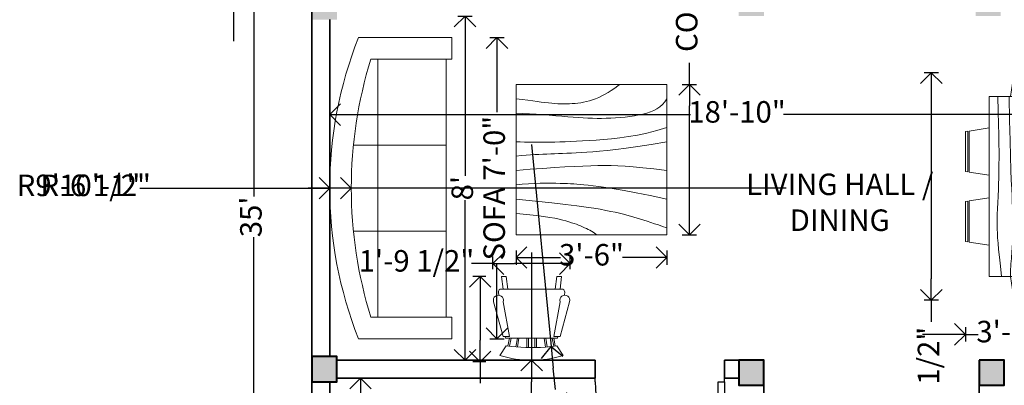
# Model space of a CAD drawing. Units: inches. Extents: x 261 to 714, y 97 to 573.
# Tile 2 of 5: x 266 to 541, y 286 to 388. Entities that reach past the tile are written whole.
import ezdxf

# ---------------------------------------------------------------- set-up
doc = ezdxf.new("R2010")
doc.units = ezdxf.units.IN
for name, color, linetype, lineweight in [('A-ANNO-DIMS', 2, 'Continuous', 18), ('A-AREA-IDEN', 7, 'Continuous', 25), ('A-COLS', 182, 'Continuous', 40), ('A-COLS-PATT', 172, 'Continuous', 13), ('A-DOOR', 182, 'Continuous', 25), ('A-FURN', 8, 'Continuous', 18), ('A-WALL', 182, 'Continuous', 35)]:
    doc.layers.add(name, color=color, linetype=linetype, lineweight=lineweight)
doc.styles.get("Standard").update_dxf_attribs({"font": 'arial.ttf'})
doc.dimstyles.new('ISO-25', dxfattribs={"dimtxt": 6, "dimasz": 6, "dimexe": 2, "dimexo": 2, "dimtad": 0, "dimdec": 1, "dimlunit": 3, "dimtxsty": 'Standard', "dimblk": 'OPEN90', "dimcen": 2.5, "dimclrd": 1, "dimclre": 1, "dimclrt": 1, "dimadec": 0, "dimazin": 0, "dimtfac": 1, "dimtdec": 1, "dimtmove": 0, "dimatfit": 3, "dimfxl": 2, "dimfxlon": 1, "dimarcsym": 0})

# ---------------------------------------------------------------- blocks, each defined once
blk = doc.blocks.new('*U4')
for p, q in [((0, 0), (0, -6)), ((36, 0), (36, -6))]:
    blk.add_line(p, q)
blk.add_lwpolyline([(0, 0), (0, 36), (1.75, 36), (1.75, 0)], close=True)
blk.add_arc((0, 0), 36, 0, 90)
blk = doc.blocks.new('_Open90')
at = {"color": 0, "linetype": 'ByBlock', "lineweight": -2}
for p, q in [((-0.5, 0.5), (0, 0)), ((0, 0), (-1, 0)), ((0, 0), (-0.5, -0.5))]:
    blk.add_line(p, q, dxfattribs=at)
blk = doc.blocks.new('*D15')
at = {"layer": 'A-ANNO-DIMS', "color": 0, "lineweight": -2, "transparency": 16777216}
for p, q in [((352.9, 361.16), (352.9, 359.16)), ((358.9, 361.16), (453.42, 361.16)), ((573.9, 361.16), (479.38, 361.16)), ((579.9, 361.16), (579.9, 359.16))]:
    blk.add_line(p, q, dxfattribs=at)
at = {"layer": 'Defpoints', "color": 0, "transparency": 16777216}
for p in [(352.9, 361.54), (579.9, 361.54), (579.9, 361.16)]:
    blk.add_point(p, dxfattribs=at)
at = {"layer": 'A-ANNO-DIMS', "color": 0, "lineweight": -2, "transparency": 16777216, "xscale": 6, "yscale": 6, "zscale": 6, "rotation": 180}
blk.add_blockref('_Open90', (352.9, 361.16), dxfattribs=at)
at = {"layer": 'A-ANNO-DIMS', "color": 0, "lineweight": -2, "transparency": 16777216, "xscale": 6, "yscale": 6, "zscale": 6}
blk.add_blockref('_Open90', (579.9, 361.16), dxfattribs=at)
at = {"layer": 'A-ANNO-DIMS', "color": 0, "transparency": 16777216, "insert": (466.4, 361.16), "char_height": 6, "attachment_point": 5}
blk.add_mtext('18\'-10"', dxfattribs=at)
blk = doc.blocks.new('*D16')
at = {"layer": 'A-ANNO-DIMS', "color": 0, "lineweight": -2, "transparency": 16777216}
for p, q in [((388.61, 388.66), (392.61, 388.66)), ((390.61, 382.66), (390.61, 344.05)), ((390.61, 298.66), (390.61, 337.27)), ((388.61, 292.66), (392.61, 292.66))]:
    blk.add_line(p, q, dxfattribs=at)
at = {"layer": 'Defpoints', "color": 0, "transparency": 16777216}
for p in [(378.75, 388.66), (378.75, 292.66), (390.61, 292.66)]:
    blk.add_point(p, dxfattribs=at)
at = {"layer": 'A-ANNO-DIMS', "color": 0, "lineweight": -2, "transparency": 16777216, "xscale": 6, "yscale": 6, "zscale": 6}
for p, rotation in [((390.61, 388.66), 90), ((390.61, 292.66), 270)]:
    blk.add_blockref('_Open90', p, dxfattribs=dict(at, rotation=rotation))
at = {"layer": 'A-ANNO-DIMS', "color": 0, "transparency": 16777216, "insert": (390.61, 340.66), "char_height": 6, "attachment_point": 5, "rotation": 90}
blk.add_mtext("8'", dxfattribs=at)
blk = doc.blocks.new('*D20')
at = {"layer": 'A-ANNO-DIMS', "color": 0, "lineweight": -2, "transparency": 16777216}
for p, q in [((363.48, 287.66), (359.48, 287.66)), ((361.48, 281.66), (361.48, 233.09)), ((361.48, 173.66), (361.48, 222.22)), ((363.48, 167.66), (359.48, 167.66))]:
    blk.add_line(p, q, dxfattribs=at)
at = {"layer": 'Defpoints', "color": 0, "transparency": 16777216}
for p in [(378.83, 287.66), (361.48, 167.66), (378.83, 167.66)]:
    blk.add_point(p, dxfattribs=at)
at = {"layer": 'A-ANNO-DIMS', "color": 0, "lineweight": -2, "transparency": 16777216, "xscale": 6, "yscale": 6, "zscale": 6}
for p, rotation in [((361.48, 287.66), 90), ((361.48, 167.66), 270)]:
    blk.add_blockref('_Open90', p, dxfattribs=dict(at, rotation=rotation))
at = {"layer": 'A-ANNO-DIMS', "color": 0, "transparency": 16777216, "insert": (361.48, 227.66), "char_height": 6, "attachment_point": 5, "rotation": 90}
blk.add_mtext("10'", dxfattribs=at)
blk = doc.blocks.new('Sofa - Roundback 7 ft.')
for p, q in [((-12.00002, -32.4421), (-12.00003, -6.5971)), ((11.99997, -32.4421), (11.99998, -6.5971)), ((-36.000027, -34), (-36.000027, -11.4696)), ((-35.999844, -13.3819), (35.9998, -13.3819)), ((35.99998, -34), (35.99998, -11.4696)), ((-36.000027, -32.4421), (35.99998, -32.4421))]:
    blk.add_line(p, q)
for points in [[(-36.000027, -34), (-42.000027, -34), (-42.000027, -8)], [(41.99998, -8), (41.99998, -34), (35.99998, -34)]]:
    blk.add_lwpolyline(points)
for centre, radius, start, end in [((0, -114.25), 114.25, 68.43141, 111.5686), ((-0.00001, -127.1968), 121.1968, 72.72033, 107.2797)]:
    blk.add_arc(centre, radius, start, end)
blk = doc.blocks.new('Table - Square Woodgrain 42 x 42 in.')
blk.add_line((0, -42), (42, -42))
for points in [[(0, -4), (1.704, -4.2172), (3.2358, -4.4188), (4.615, -4.604), (5.8615, -4.7721), (6.9951, -4.9224), (8.0357, -5.0541), (9.0031, -5.1667), (9.9171, -5.2594), (10.7951, -5.3316), (11.6445, -5.3836), (12.4702, -5.4157), (13.277, -5.4283), (14.0698, -5.4217), (14.8535, -5.3964), (15.6331, -5.3526), (16.4133, -5.2908), (17.1986, -5.2103), (17.9913, -5.1062), (18.793, -4.9727), (19.6056, -4.8038), (20.4307, -4.5937), (21.2701, -4.3365), (22.1256, -4.0262), (22.9989, -3.6571), (23.888, -3.2272), (24.7756, -2.7516), (25.6408, -2.2491), (26.4624, -1.7387), (27.2195, -1.2395), (27.891, -0.7703), (28.456, -0.3501), (28.8934, 0.002)], [(0, -42), (0, 0), (42, 0), (42, -42)], [(0, -8), (1.8203, -8.1001), (3.6741, -8.2149), (5.5411, -8.3408), (7.4011, -8.4741), (9.2339, -8.6112), (11.0193, -8.7484), (12.7371, -8.8821), (14.3671, -9.0086), (15.8954, -9.1246), (17.3337, -9.2278), (18.6997, -9.3159), (20.0116, -9.387), (21.2871, -9.4389), (22.5442, -9.4696), (23.8008, -9.477), (25.0749, -9.459), (26.3791, -9.4137), (27.7049, -9.3403), (29.0383, -9.2382), (30.3655, -9.1068), (31.6728, -8.9455), (32.9461, -8.7535), (34.1717, -8.5304), (35.3358, -8.2756), (36.4268, -7.9863), (37.443, -7.6521), (38.3849, -7.2603), (39.253, -6.7986), (40.048, -6.2542), (40.7705, -5.6147), (41.421, -4.8674), (42, -4)], [(42, -12), (39.1784, -12.8621), (36.4519, -13.5654), (33.8246, -14.1294), (31.3004, -14.5731), (28.8832, -14.9161), (26.577, -15.1775), (24.3858, -15.3768), (22.3136, -15.5332), (20.3622, -15.6632), (18.5254, -15.7718), (16.7947, -15.8612), (15.1618, -15.9338), (13.6183, -15.9916), (12.1558, -16.0369), (10.7659, -16.0718), (9.4403, -16.0987), (8.1703, -16.1191), (6.9461, -16.1325), (5.7577, -16.1377), (4.595, -16.1335), (3.4479, -16.1188), (2.3064, -16.0924), (1.1604, -16.0532), (0, -16)], [(42, -16), (37.6529, -16.7365), (33.8802, -17.329), (30.6179, -17.7961), (27.8015, -18.1561), (25.3668, -18.4275), (23.2497, -18.6288), (21.3859, -18.7785), (19.7111, -18.8949), (18.1693, -18.9939), (16.7375, -19.0795), (15.401, -19.1534), (14.1449, -19.217), (12.9544, -19.2717), (11.8148, -19.3191), (10.7113, -19.3606), (9.6291, -19.3976), (8.5534, -19.4323), (7.47, -19.4689), (6.3643, -19.5122), (5.222, -19.5672), (4.0288, -19.6386), (2.7703, -19.7313), (1.4321, -19.8501), (0, -20)], [(0, -24), (3.9243, -23.6805), (7.4766, -23.4138), (10.6891, -23.1954), (13.5943, -23.0205), (16.2247, -22.8847), (18.6125, -22.7832), (20.7903, -22.7116), (22.7903, -22.6651), (24.6563, -22.642), (26.4764, -22.6507), (28.35, -22.7024), (30.3766, -22.8084), (32.6555, -22.98), (35.2861, -23.2283), (38.3678, -23.5645), (42, -24)], [(42, -32), (37.392, -31.017), (33.4585, -30.2231), (30.1291, -29.5949), (27.3334, -29.109), (25.0009, -28.742), (23.0612, -28.4707), (21.4439, -28.2716), (20.0786, -28.1215), (18.8998, -28.0002), (17.8609, -27.9014), (16.9206, -27.8219), (16.0371, -27.7588), (15.1691, -27.709), (14.2748, -27.6693), (13.3128, -27.6368), (12.2415, -27.6083), (11.0295, -27.5824), (9.6867, -27.5643), (8.233, -27.5608), (6.6884, -27.5787), (5.0728, -27.6248), (3.4062, -27.7058), (1.7086, -27.8286), (0, -28)], [(0, -32), (5.4026, -32.5358), (9.9494, -33.019), (13.7424, -33.4553), (16.8834, -33.8505), (19.4743, -34.2106), (21.6171, -34.5413), (23.4136, -34.8486), (24.9657, -35.1382), (26.3614, -35.4156), (27.6332, -35.6841), (28.7995, -35.9467), (29.8788, -36.2064), (30.8897, -36.4661), (31.8507, -36.7288), (32.7802, -36.9973), (33.6968, -37.2747), (34.6175, -37.5635), (35.5531, -37.8651), (36.5128, -38.1805), (37.506, -38.5108), (38.5421, -38.8568), (39.6302, -39.2197), (40.7797, -39.6004), (42, -40)], [(0, -36), (3.0098, -36.2857), (5.5354, -36.5643), (7.6368, -36.8359), (9.374, -37.1009), (10.807, -37.3597), (11.9957, -37.6126), (13.0002, -37.8599), (13.8804, -38.102), (14.6874, -38.3393), (15.4365, -38.5729), (16.1338, -38.8041), (16.7858, -39.0341), (17.3987, -39.264), (17.9787, -39.4952), (18.5322, -39.7288), (19.0655, -39.9662), (19.5832, -40.2081), (20.0842, -40.4544), (20.5657, -40.7046), (21.0249, -40.9581), (21.459, -41.2144), (21.8653, -41.4731), (22.2409, -41.7335), (22.5831, -41.9951)]]:
    blk.add_lwpolyline(points)
blk = doc.blocks.new('Dining Set - 36 x 72 in.')
for p, q in [((-22.2343, 26.00059), (-23.4847, 17.99762)), ((-22.2304, 26), (-5.7608, 26)), ((-22, 27.5), (-22.1562, 26.50042)), ((-5.8416, 26.5), (-22.1534, 26.5)), ((-22, 27.5), (-6, 27.5)), ((-5.8437, 26.49966), (-6, 27.5)), ((-4.5152, 17.99762), (-5.7655, 25.99926)), ((5.7657, 26.00059), (4.5153, 17.99762)), ((5.7696, 26), (22.2392, 26)), ((6, 27.5), (5.8438, 26.50042)), ((22.1584, 26.5), (5.8466, 26.5)), ((6, 27.5), (22, 27.5)), ((22.1563, 26.49966), (22, 27.5)), ((23.4848, 17.99762), (22.2345, 25.99926)), ((36, 18), (-36, 18)), ((-36, 18), (-36, -18)), ((36, -18), (36, 18)), ((-45.5, 8), (-44.5004, 8.15617)), ((-45.5, 8), (-45.5, -8)), ((-44.5, -8.15843), (-44.5, 8.15338)), ((-44.0006, 8.23428), (-35.9976, 9.48474)), ((-44, 8.23041), (-44, -8.23915)), ((44.0006, 8.23428), (35.9976, 9.48474)), ((44, 8.23041), (44, -8.23915)), ((44.5, -8.15843), (44.5, 8.15338)), ((45.5, 8), (44.5005, 8.15617)), ((45.5, 8), (45.5, -8)), ((-44.4997, -8.15631), (-45.5, -8)), ((-35.9976, -9.48476), (-43.9993, -8.2345)), ((35.9976, -9.48476), (43.9993, -8.2345)), ((44.4997, -8.15631), (45.5, -8)), ((-36, -18), (36, -18)), ((-22.2343, -26.0006), (-23.4847, -17.99762)), ((-4.5152, -17.99762), (-5.7655, -25.99928)), ((5.7657, -26.0006), (4.5153, -17.99762)), ((23.4848, -17.99762), (22.2345, -25.99928)), ((-22.2304, -26), (-5.7608, -26)), ((-22, -27.5), (-22.1562, -26.50044)), ((-5.8416, -26.5), (-22.1534, -26.5)), ((-22, -27.5), (-6, -27.5)), ((-5.8437, -26.49967), (-6, -27.5)), ((5.7696, -26), (22.2392, -26)), ((6, -27.5), (5.8438, -26.50044)), ((22.1584, -26.5), (5.8466, -26.5)), ((6, -27.5), (22, -27.5)), ((22.1563, -26.49967), (22, -27.5))]:
    blk.add_line(p, q)
for points in [[(-36, 15), (-31.1772, 14.97754), (-26.8079, 14.91406), (-22.8538, 14.81543), (-19.276, 14.6875), (-16.0362, 14.53613), (-13.0957, 14.36718), (-10.4159, 14.18652), (-7.9583, 14), (-5.6904, 13.81315), (-3.6035, 13.63021), (-1.6954, 13.45508), (0.0365, 13.29166), (1.5945, 13.14388), (2.9811, 13.01562), (4.1988, 12.9108), (5.25, 12.83333), (6.1393, 12.78613), (6.8802, 12.76823), (7.4883, 12.77767), (7.9792, 12.8125), (8.3685, 12.87077), (8.6719, 12.95052), (8.9049, 13.0498), (9.0833, 13.16666), (9.2205, 13.29899), (9.3216, 13.44401), (9.3895, 13.59879), (9.4271, 13.76041), (9.4373, 13.92594), (9.4232, 14.09245), (9.3875, 14.257), (9.3333, 14.41666), (9.2638, 14.56917), (9.1836, 14.71484), (9.0975, 14.85465), (9.0104, 14.98958), (8.9272, 15.1206), (8.8529, 15.2487), (8.7922, 15.37483), (8.75, 15.5), (8.7305, 15.62467), (8.7344, 15.74739), (8.7617, 15.86621), (8.8125, 15.97916), (8.8867, 16.08431), (8.9844, 16.17968), (9.1055, 16.26334), (9.25, 16.33333), (9.4189, 16.38802), (9.6172, 16.42708), (9.8506, 16.45052), (10.125, 16.45833), (10.4463, 16.45052), (10.8203, 16.42708), (11.2529, 16.38802), (11.75, 16.33333), (12.3184, 16.26318), (12.9694, 16.17838), (13.7151, 16.07991), (14.5677, 15.96875), (15.5395, 15.84586), (16.6426, 15.71224), (17.8893, 15.56884), (19.2917, 15.41666), (20.859, 15.25667), (22.5879, 15.08984), (24.4721, 14.91715), (26.5052, 14.73958), (28.6809, 14.5581), (30.9929, 14.3737), (33.4347, 14.18733), (36, 14)], [(-36, 10), (-28.9766, 10.14274), (-23.1725, 10.20442), (-18.4241, 10.19775), (-14.5677, 10.13541), (-11.4399, 10.03011), (-8.877, 9.89453), (-6.7154, 9.74137), (-4.7917, 9.58333), (-2.9698, 9.43082), (-1.2246, 9.28515), (0.4415, 9.14534), (2.026, 9.01041), (3.5266, 8.87939), (4.9408, 8.7513), (6.266, 8.62516), (7.5, 8.5), (8.6411, 8.37549), (9.6914, 8.2539), (10.6538, 8.13818), (11.5312, 8.03125), (12.3267, 7.93603), (13.043, 7.85547), (13.6831, 7.79248), (14.25, 7.75), (14.7471, 7.7303), (15.1797, 7.73307), (15.5537, 7.75732), (15.875, 7.80208), (16.1494, 7.86637), (16.3828, 7.94922), (16.5811, 8.04964), (16.75, 8.16666), (16.8944, 8.29915), (17.0143, 8.44531), (17.1089, 8.60319), (17.1771, 8.77083), (17.218, 8.94629), (17.2305, 9.1276), (17.2137, 9.31282), (17.1667, 9.5), (17.0895, 9.6875), (16.987, 9.875), (16.8649, 10.0625), (16.7292, 10.25), (16.5856, 10.4375), (16.4401, 10.625), (16.2985, 10.8125), (16.1667, 11), (16.05, 11.18733), (15.9518, 11.3737), (15.8752, 11.5581), (15.8229, 11.73958), (15.798, 11.91715), (15.8034, 12.08984), (15.842, 12.25667), (15.9167, 12.41666), (16.0295, 12.56836), (16.1784, 12.70833), (16.3605, 12.83268), (16.5729, 12.9375), (16.8127, 13.01888), (17.0768, 13.07291), (17.3625, 13.0957), (17.6667, 13.08333), (17.9894, 13.03312), (18.3418, 12.94726), (18.7382, 12.82918), (19.1927, 12.68229), (19.7195, 12.51001), (20.3327, 12.31575), (21.0465, 12.10294), (21.875, 11.875), (22.8357, 11.63354), (23.959, 11.37304), (25.2786, 11.08618), (26.8282, 10.76562), (28.6414, 10.40405), (30.752, 9.99414), (33.1936, 9.52856), (36, 9)], [(-36, 5.5), (-30.7157, 5.3348), (-26.069, 5.20963), (-21.9946, 5.11767), (-18.4271, 5.05208), (-15.3009, 5.00602), (-12.5508, 4.97265), (-10.1112, 4.94515), (-7.9167, 4.91666), (-5.909, 4.88167), (-4.0586, 4.83984), (-2.3429, 4.79215), (-0.7396, 4.73958), (0.7739, 4.6831), (2.22, 4.6237), (3.6213, 4.56233), (5, 4.5), (6.373, 4.43782), (7.7344, 4.3776), (9.0723, 4.32129), (10.375, 4.27083), (11.6309, 4.22819), (12.8281, 4.19531), (13.9551, 4.17415), (15, 4.16666), (15.954, 4.17448), (16.819, 4.19791), (17.6001, 4.23698), (18.3021, 4.29166), (18.9299, 4.36198), (19.4883, 4.44791), (19.9823, 4.54948), (20.4167, 4.66666), (20.7969, 4.79899), (21.1302, 4.94401), (21.4245, 5.09879), (21.6875, 5.26041), (21.9271, 5.42594), (22.1511, 5.59245), (22.3672, 5.757), (22.5834, 5.91666), (22.8065, 6.06868), (23.0404, 6.21093), (23.2879, 6.34147), (23.5521, 6.45833), (23.8358, 6.55957), (24.142, 6.64323), (24.4735, 6.70735), (24.8334, 6.75), (25.2235, 6.76969), (25.642, 6.76692), (26.0858, 6.74267), (26.5521, 6.69791), (27.0379, 6.63362), (27.5404, 6.55078), (28.0565, 6.45036), (28.5834, 6.33333), (29.1242, 6.19987), (29.7071, 6.04687), (30.3661, 5.87044), (31.1354, 5.66666), (32.0493, 5.43164), (33.142, 5.16146), (34.4475, 4.85221), (36, 4.5)], [(-36, -1), (-30.7915, -0.6591), (-26.0195, -0.38216), (-21.6519, -0.16284), (-17.6563, 0.00521), (-14.0005, 0.12833), (-10.6523, 0.21289), (-7.5796, 0.26522), (-4.75, 0.29166), (-2.134, 0.29793), (0.2878, 0.28711), (2.5317, 0.26163), (4.6146, 0.22396), (6.5529, 0.17651), (8.3633, 0.12174), (10.0623, 0.06209), (11.6667, 0), (13.1899, -0.06201), (14.6341, -0.1211), (15.9982, -0.17432), (17.2813, -0.21875), (18.4823, -0.25147), (19.6003, -0.26953), (20.6343, -0.27002), (21.5834, -0.25), (22.4481, -0.20768), (23.2357, -0.14584), (23.9549, -0.06836), (24.6146, 0.02083), (25.2235, 0.11784), (25.7904, 0.21875), (26.3241, 0.31966), (26.8334, 0.41666), (27.3265, 0.50618), (27.8099, 0.58593), (28.2894, 0.65397), (28.7709, 0.70833), (29.2601, 0.74707), (29.763, 0.76823), (30.2855, 0.76985), (30.8334, 0.75), (31.4088, 0.70784), (31.9994, 0.64713), (32.589, 0.57275), (33.1615, 0.48958), (33.7008, 0.4025), (34.1908, 0.3164), (34.6153, 0.23616), (34.9584, 0.16666), (35.2099, 0.11165), (35.3848, 0.07031), (35.504, 0.04069), (35.5886, 0.02083), (35.6594, 0.00879), (35.7377, 0.0026), (35.8442, 0.00032), (36, 0)], [(-36, -6.5), (-27.1843, -6.31267), (-20.084, -6.1263), (-14.469, -5.9419), (-10.1094, -5.76042), (-6.7752, -5.58285), (-4.2363, -5.41016), (-2.2629, -5.24333), (-0.625, -5.08334), (0.8708, -4.93099), (2.2715, -4.78646), (3.5872, -4.64974), (4.8281, -4.52084), (6.0046, -4.39974), (7.127, -4.28646), (8.2053, -4.18099), (9.25, -4.08334), (10.2705, -3.99382), (11.2734, -3.91407), (12.2647, -3.84603), (13.25, -3.79167), (14.2354, -3.75293), (15.2266, -3.73177), (16.2295, -3.73015), (17.25, -3.75), (18.2912, -3.79248), (19.3451, -3.85547), (20.4009, -3.93604), (21.4479, -4.03125), (22.4754, -4.13819), (23.4727, -4.25391), (24.4289, -4.37549), (25.3334, -4.5), (26.1785, -4.62492), (26.9694, -4.74935), (27.7145, -4.87281), (28.4219, -4.99479), (29.1, -5.11483), (29.7572, -5.23242), (30.4016, -5.34709), (31.0417, -5.45834), (31.6837, -5.56437), (32.3262, -5.65821), (32.9658, -5.73153), (33.599, -5.77604), (34.2224, -5.78345), (34.8327, -5.74545), (35.4264, -5.65373), (36, -5.5)], [(-36, -10), (-26.4022, -9.81299), (-18.4675, -9.62891), (-11.9839, -9.45069), (-6.7396, -9.28125), (-2.5226, -9.12354), (0.8789, -8.98047), (3.6769, -8.85498), (6.0833, -8.75), (8.2767, -8.66765), (10.3021, -8.60677), (12.1712, -8.56543), (13.8958, -8.54167), (15.4876, -8.53353), (16.9583, -8.53907), (18.3197, -8.55632), (19.5834, -8.58334), (20.7616, -8.61841), (21.8685, -8.66081), (22.9188, -8.71004), (23.9271, -8.76563), (24.9081, -8.82707), (25.8763, -8.89388), (26.8465, -8.96558), (27.8334, -9.04167), (28.8474, -9.12118), (29.8828, -9.20117), (30.93, -9.27824), (31.9792, -9.34896), (33.0205, -9.40991), (34.0443, -9.45768), (35.0407, -9.48885), (36, -9.5)], [(-36, -14.5), (-30.0881, -14.33513), (-25.0332, -14.21224), (-20.7312, -14.12647), (-17.0781, -14.07292), (-13.97, -14.04671), (-11.3027, -14.04297), (-8.9724, -14.05681), (-6.875, -14.08334), (-4.9224, -14.11833), (-3.0905, -14.16016), (-1.3709, -14.20785), (0.2448, -14.26042), (1.7647, -14.3169), (3.1973, -14.3763), (4.5507, -14.43767), (5.8333, -14.5), (7.0554, -14.5621), (8.235, -14.62175), (9.3922, -14.67652), (10.5469, -14.72396), (11.7192, -14.76164), (12.929, -14.78711), (14.1965, -14.79794), (15.5417, -14.79167), (16.9933, -14.76424), (18.6152, -14.70508), (20.4804, -14.60197), (22.6615, -14.44271), (25.2312, -14.21509), (28.2624, -13.9069), (31.8277, -13.50594), (36, -13)]]:
    blk.add_lwpolyline(points)
blk = doc.blocks.new('Chair - Rocking')
for p, q in [((-8, -4.5), (-10, -1.5)), ((8, -4.5), (10, -1.5)), ((-7.5, -4.5), (-7, -7)), ((-6.5, -7), (-7.02225, -4.43)), ((-4.5, -7), (-4.96674, -4.19951)), ((-4, -7), (-4.40532, -4.16272)), ((-1.5, -4.05012), (-1.5, -7)), ((-1, -7), (-1, -4.05012)), ((1, -7), (1, -4.04655)), ((1.5, -4.05012), (1.5, -7)), ((4, -7), (4.40187, -4.18694)), ((4.5, -7), (4.96761, -4.19437)), ((6.5, -7), (7, -4.4057)), ((7.5, -4.5), (7, -7)), ((-9, -7.5), (-12, -18.49999)), ((-7, -7.5), (-9, -7.5)), ((-9, -18.49999), (-7, -7.5)), ((-8.23428, -6.99939), (-8.3093, -7.47958)), ((-8.23041, -7), (8.23915, -7)), ((7, -7.5), (9, -7.5)), ((9, -18.49999), (7, -7.5)), ((8.31071, -7.48854), (8.23449, -7.00073)), ((9, -7.5), (12, -18.49999)), ((-10.36644, -20.64523), (-10.5, -21.49999)), ((10.5, -21.49999), (10.3575, -20.58798)), ((-9, -22.49999), (-9.5, -26.49999)), ((0, -22.49999), (-9.5, -22.49999)), ((-8, -26.49999), (-7.5, -22.49999)), ((0, -22.49999), (9.5, -22.49999)), ((8, -26.49999), (7.5, -22.49999)), ((9, -22.49999), (9.5, -26.49999)), ((-9.5, -26.49999), (-8, -26.49999)), ((9.5, -26.49999), (8, -26.49999))]:
    blk.add_line(p, q)
for centre, radius, start, end in [((0, -34.08333), 34.08333, 72.93847, 107.0615), ((0, -68.25004), 64.25, 93.92211, 97.15267), ((0, -68.25004), 64.25, 82.84733, 93.92211), ((-10.5, -18.99999), 1.58114, 161.5651, 18.43495), ((10.5, -18.99999), 1.58114, 161.5651, 18.43495), ((-9.5, -21.49999), 1, 180, 270), ((9.5, -21.49999), 1, 270, 0)]:
    blk.add_arc(centre, radius, start, end)
blk = doc.blocks.new('*D36')
at = {"layer": 'A-ANNO-DIMS', "color": 0, "lineweight": -2, "transparency": 16777216}
for p, q in [((333.7, 542.66), (329.7, 542.66)), ((331.7, 536.66), (331.7, 338.37)), ((331.7, 128.66), (331.7, 326.94)), ((333.7, 122.66), (329.7, 122.66))]:
    blk.add_line(p, q, dxfattribs=at)
at = {"layer": 'Defpoints', "color": 0, "transparency": 16777216}
for p in [(347.9, 542.66), (331.7, 122.66), (347.9, 122.66)]:
    blk.add_point(p, dxfattribs=at)
at = {"layer": 'A-ANNO-DIMS', "color": 0, "lineweight": -2, "transparency": 16777216, "xscale": 6, "yscale": 6, "zscale": 6}
for p, rotation in [((331.7, 542.66), 90), ((331.7, 122.66), 270)]:
    blk.add_blockref('_Open90', p, dxfattribs=dict(at, rotation=rotation))
at = {"layer": 'A-ANNO-DIMS', "color": 0, "transparency": 16777216, "insert": (331.7, 332.66), "char_height": 6, "attachment_point": 5, "rotation": 90}
blk.add_mtext("35'", dxfattribs=at)
blk = doc.blocks.new('COLUMN-7IN-SQUARE')
blk.add_lwpolyline([(0, 7), (0, 2), (0, 0), (2, 0), (7, 0), (7, 2), (7, 7)], close=True)
blk = doc.blocks.new('*D45')
at = {"layer": 'A-ANNO-DIMS', "color": 1, "lineweight": -2, "transparency": 16777216}
for p, q in [((397.5, 382.66), (401.5, 382.66)), ((399.5, 376.66), (399.5, 361.82)), ((399.5, 304.66), (399.5, 319.5)), ((397.5, 298.66), (401.5, 298.66))]:
    blk.add_line(p, q, dxfattribs=at)
at = {"layer": 'Defpoints', "color": 0, "transparency": 16777216}
for p in [(386.9, 382.66), (399.5, 382.66), (386.9, 298.66)]:
    blk.add_point(p, dxfattribs=at)
at = {"layer": 'A-ANNO-DIMS', "color": 1, "lineweight": -2, "transparency": 16777216, "xscale": 6, "yscale": 6, "zscale": 6}
for p, rotation in [((399.5, 382.66), 90), ((399.5, 298.66), 270)]:
    blk.add_blockref('_Open90', p, dxfattribs=dict(at, rotation=rotation))
at = {"layer": 'A-ANNO-DIMS', "color": 1, "transparency": 16777216, "insert": (399.5, 340.66), "char_height": 6, "attachment_point": 5, "rotation": 90}
blk.add_mtext('SOFA 7\'-0"', dxfattribs=at)
blk = doc.blocks.new('*D46')
at = {"layer": 'A-ANNO-DIMS', "color": 1, "lineweight": -2, "transparency": 16777216}
for p, q in [((344.24, 395.26), (338.24, 395.26)), ((350.24, 393.26), (350.24, 397.26)), ((350.24, 395.26), (352.98, 395.26)), ((386.9, 395.26), (384.16, 395.26)), ((386.9, 393.26), (386.9, 397.26)), ((392.9, 395.26), (398.9, 395.26))]:
    blk.add_line(p, q, dxfattribs=at)
at = {"layer": 'Defpoints', "color": 0, "transparency": 16777216}
for p in [(350.24, 395.26), (350.24, 382.66), (386.9, 382.66)]:
    blk.add_point(p, dxfattribs=at)
at = {"layer": 'A-ANNO-DIMS', "color": 1, "lineweight": -2, "transparency": 16777216, "xscale": 6, "yscale": 6, "zscale": 6}
blk.add_blockref('_Open90', (350.24, 395.26), dxfattribs=at)
at = {"layer": 'A-ANNO-DIMS', "color": 1, "lineweight": -2, "transparency": 16777216, "xscale": 6, "yscale": 6, "zscale": 6, "rotation": 180}
blk.add_blockref('_Open90', (386.9, 395.26), dxfattribs=at)
at = {"layer": 'A-ANNO-DIMS', "color": 1, "transparency": 16777216, "insert": (368.57, 395.26), "char_height": 6, "attachment_point": 5}
blk.add_mtext('3\'-0 1/2"', dxfattribs=at)
blk = doc.blocks.new('*D47')
at = {"layer": 'A-ANNO-DIMS', "color": 1, "lineweight": -2, "transparency": 16777216}
for p, q in [((453.15, 369.61), (453.15, 375.61)), ((451.15, 369.61), (455.15, 369.61)), ((453.15, 333.6), (453.15, 363.61)), ((451.15, 327.6), (455.15, 327.6))]:
    blk.add_line(p, q, dxfattribs=at)
at = {"layer": 'Defpoints', "color": 0, "transparency": 16777216}
for p in [(446.85, 369.61), (453.15, 369.61), (446.85, 327.6)]:
    blk.add_point(p, dxfattribs=at)
at = {"layer": 'A-ANNO-DIMS', "color": 1, "lineweight": -2, "transparency": 16777216, "xscale": 6, "yscale": 6, "zscale": 6}
for p, rotation in [((453.15, 369.61), 90), ((453.15, 327.6), 270)]:
    blk.add_blockref('_Open90', p, dxfattribs=dict(at, rotation=rotation))
at = {"layer": 'A-ANNO-DIMS', "color": 1, "transparency": 16777216, "insert": (453.15, 416.77), "char_height": 6, "attachment_point": 5, "rotation": 90}
blk.add_mtext('COFFEE TABLE 3\'-6"', dxfattribs=at)
blk = doc.blocks.new('*D48')
at = {"layer": 'A-ANNO-DIMS', "color": 1, "lineweight": -2, "transparency": 16777216}
for p, q in [((404.85, 323.3), (404.85, 319.3)), ((410.85, 321.3), (417.25, 321.3)), ((440.85, 321.3), (434.45, 321.3)), ((446.85, 323.3), (446.85, 319.3))]:
    blk.add_line(p, q, dxfattribs=at)
at = {"layer": 'Defpoints', "color": 0, "transparency": 16777216}
for p in [(404.85, 327.6), (446.85, 327.6), (446.85, 321.3)]:
    blk.add_point(p, dxfattribs=at)
at = {"layer": 'A-ANNO-DIMS', "color": 1, "lineweight": -2, "transparency": 16777216, "xscale": 6, "yscale": 6, "zscale": 6, "rotation": 180}
blk.add_blockref('_Open90', (404.85, 321.3), dxfattribs=at)
at = {"layer": 'A-ANNO-DIMS', "color": 1, "lineweight": -2, "transparency": 16777216, "xscale": 6, "yscale": 6, "zscale": 6}
blk.add_blockref('_Open90', (446.85, 321.3), dxfattribs=at)
at = {"layer": 'A-ANNO-DIMS', "color": 1, "transparency": 16777216, "insert": (425.85, 321.3), "char_height": 6, "attachment_point": 5}
blk.add_mtext('3\'-6"', dxfattribs=at)
blk = doc.blocks.new('*D51')
at = {"layer": 'A-ANNO-DIMS', "color": 1, "lineweight": -2, "transparency": 16777216}
for p, q in [((522.54, 372.81), (518.54, 372.81)), ((520.54, 366.81), (520.54, 315.39)), ((522.54, 309.39), (518.54, 309.39)), ((520.54, 309.39), (520.54, 303.39))]:
    blk.add_line(p, q, dxfattribs=at)
at = {"layer": 'Defpoints', "color": 0, "transparency": 16777216}
for p in [(530.06, 372.81), (520.54, 309.39), (530.06, 309.39)]:
    blk.add_point(p, dxfattribs=at)
at = {"layer": 'A-ANNO-DIMS', "color": 1, "lineweight": -2, "transparency": 16777216, "xscale": 6, "yscale": 6, "zscale": 6}
for p, rotation in [((520.54, 372.81), 90), ((520.54, 309.39), 270)]:
    blk.add_blockref('_Open90', p, dxfattribs=dict(at, rotation=rotation))
at = {"layer": 'A-ANNO-DIMS', "color": 1, "transparency": 16777216, "insert": (520.54, 262.8), "char_height": 6, "attachment_point": 5, "rotation": 90}
blk.add_mtext('DINING SET 5\'-3 1/2"', dxfattribs=at)
blk = doc.blocks.new('*D52')
at = {"layer": 'A-ANNO-DIMS', "color": 1, "lineweight": -2, "transparency": 16777216}
for p, q in [((530.06, 301.87), (530.06, 297.87)), ((568.39, 301.87), (568.39, 297.87)), ((524.06, 299.87), (518.06, 299.87)), ((530.06, 299.87), (533.63, 299.87)), ((568.39, 299.87), (564.81, 299.87)), ((574.39, 299.87), (580.39, 299.87))]:
    blk.add_line(p, q, dxfattribs=at)
at = {"layer": 'Defpoints', "color": 0, "transparency": 16777216}
for p in [(530.06, 309.39), (568.39, 309.39), (568.39, 299.87)]:
    blk.add_point(p, dxfattribs=at)
at = {"layer": 'A-ANNO-DIMS', "color": 1, "lineweight": -2, "transparency": 16777216, "xscale": 6, "yscale": 6, "zscale": 6}
blk.add_blockref('_Open90', (530.06, 299.87), dxfattribs=at)
at = {"layer": 'A-ANNO-DIMS', "color": 1, "lineweight": -2, "transparency": 16777216, "xscale": 6, "yscale": 6, "zscale": 6, "rotation": 180}
blk.add_blockref('_Open90', (568.39, 299.87), dxfattribs=at)
at = {"layer": 'A-ANNO-DIMS', "color": 1, "transparency": 16777216, "insert": (549.22, 299.87), "char_height": 6, "attachment_point": 5}
blk.add_mtext('3\'-2 1/2"', dxfattribs=at)
blk = doc.blocks.new('*D53')
at = {"layer": 'A-ANNO-DIMS', "color": 1, "lineweight": -2, "transparency": 16777216}
for p, q in [((396.37, 316.03), (392.8, 316.03)), ((394.8, 310.03), (394.8, 298.22)), ((396.37, 292.22), (392.8, 292.22)), ((394.8, 292.22), (394.8, 286.22))]:
    blk.add_line(p, q, dxfattribs=at)
at = {"layer": 'Defpoints', "color": 0, "transparency": 16777216}
for p in [(398.37, 316.03), (394.8, 292.22), (398.37, 292.22)]:
    blk.add_point(p, dxfattribs=at)
at = {"layer": 'A-ANNO-DIMS', "color": 1, "lineweight": -2, "transparency": 16777216, "xscale": 6, "yscale": 6, "zscale": 6}
for p, rotation in [((394.8, 316.03), 90), ((394.8, 292.22), 270)]:
    blk.add_blockref('_Open90', p, dxfattribs=dict(at, rotation=rotation))
at = {"layer": 'A-ANNO-DIMS', "color": 1, "transparency": 16777216, "insert": (394.8, 242.84), "char_height": 6, "attachment_point": 5, "rotation": 90}
blk.add_mtext('ROCKING CHAIR 2\'-0"', dxfattribs=at)
blk = doc.blocks.new('*D54')
at = {"layer": 'A-ANNO-DIMS', "color": 1, "lineweight": -2, "transparency": 16777216}
for p, q in [((398.37, 318.03), (398.37, 321.6)), ((419.93, 318.03), (419.93, 321.6)), ((398.37, 319.6), (392.37, 319.6)), ((413.93, 319.6), (404.37, 319.6))]:
    blk.add_line(p, q, dxfattribs=at)
at = {"layer": 'Defpoints', "color": 0, "transparency": 16777216}
for p in [(398.37, 319.6), (398.37, 316.03), (419.93, 316.03)]:
    blk.add_point(p, dxfattribs=at)
at = {"layer": 'A-ANNO-DIMS', "color": 1, "lineweight": -2, "transparency": 16777216, "xscale": 6, "yscale": 6, "zscale": 6, "rotation": 180}
blk.add_blockref('_Open90', (398.37, 319.6), dxfattribs=at)
at = {"layer": 'A-ANNO-DIMS', "color": 1, "lineweight": -2, "transparency": 16777216, "xscale": 6, "yscale": 6, "zscale": 6}
blk.add_blockref('_Open90', (419.93, 319.6), dxfattribs=at)
at = {"layer": 'A-ANNO-DIMS', "color": 1, "transparency": 16777216, "insert": (377.07, 319.6), "char_height": 6, "attachment_point": 5}
blk.add_mtext('1\'-9 1/2"', dxfattribs=at)
blk = doc.blocks.new('*D61')
at = {"layer": 'A-ANNO-DIMS', "color": 1, "lineweight": -2, "transparency": 16777216}
for p, q in [((354.9, 102.81), (354.9, 98.81)), ((426.9, 102.81), (426.9, 98.81)), ((360.9, 100.81), (382.29, 100.81)), ((420.9, 100.81), (399.52, 100.81))]:
    blk.add_line(p, q, dxfattribs=at)
at = {"layer": 'Defpoints', "color": 0, "transparency": 16777216}
for p in [(354.9, 287.66), (426.9, 287.66), (426.9, 100.81)]:
    blk.add_point(p, dxfattribs=at)
at = {"layer": 'A-ANNO-DIMS', "color": 1, "lineweight": -2, "transparency": 16777216, "xscale": 6, "yscale": 6, "zscale": 6, "rotation": 180}
blk.add_blockref('_Open90', (354.9, 100.81), dxfattribs=at)
at = {"layer": 'A-ANNO-DIMS', "color": 1, "lineweight": -2, "transparency": 16777216, "xscale": 6, "yscale": 6, "zscale": 6}
blk.add_blockref('_Open90', (426.9, 100.81), dxfattribs=at)
at = {"layer": 'A-ANNO-DIMS', "color": 1, "transparency": 16777216, "insert": (390.9, 100.81), "char_height": 6, "attachment_point": 5}
blk.add_mtext('6\'-0"', dxfattribs=at)
blk = doc.blocks.new('*D62')
at = {"layer": 'A-ANNO-DIMS', "color": 1, "lineweight": -2, "transparency": 16777216}
for p, q in [((426.9, 102.81), (426.9, 98.81)), ((462.9, 102.81), (462.9, 98.81)), ((432.9, 100.81), (436.31, 100.81)), ((456.9, 100.81), (453.5, 100.81))]:
    blk.add_line(p, q, dxfattribs=at)
at = {"layer": 'Defpoints', "color": 0, "transparency": 16777216}
for p in [(426.9, 287.66), (462.9, 287.66), (462.9, 100.81)]:
    blk.add_point(p, dxfattribs=at)
at = {"layer": 'A-ANNO-DIMS', "color": 1, "lineweight": -2, "transparency": 16777216, "xscale": 6, "yscale": 6, "zscale": 6, "rotation": 180}
blk.add_blockref('_Open90', (426.9, 100.81), dxfattribs=at)
at = {"layer": 'A-ANNO-DIMS', "color": 1, "lineweight": -2, "transparency": 16777216, "xscale": 6, "yscale": 6, "zscale": 6}
blk.add_blockref('_Open90', (462.9, 100.81), dxfattribs=at)
at = {"layer": 'A-ANNO-DIMS', "color": 1, "transparency": 16777216, "insert": (444.9, 100.81), "char_height": 6, "attachment_point": 5}
blk.add_mtext('3\'-0"', dxfattribs=at)
blk = doc.blocks.new('*D74')
at = {"layer": 'A-ANNO-DIMS', "color": 1, "lineweight": -2, "transparency": 16777216}
for p, q in [((326.05, 417.65), (326.05, 423.65)), ((328.05, 411.65), (324.05, 411.65)), ((326.05, 411.65), (326.05, 410.97)), ((328.05, 393.66), (324.05, 393.66)), ((326.05, 393.66), (326.05, 394.34)), ((326.05, 387.66), (326.05, 381.66))]:
    blk.add_line(p, q, dxfattribs=at)
at = {"layer": 'Defpoints', "color": 0, "transparency": 16777216}
for p in [(326.05, 411.65), (417.18, 411.65), (417.18, 393.66)]:
    blk.add_point(p, dxfattribs=at)
at = {"layer": 'A-ANNO-DIMS', "color": 1, "lineweight": -2, "transparency": 16777216, "xscale": 6, "yscale": 6, "zscale": 6}
for p, rotation in [((326.05, 411.65), 270), ((326.05, 393.66), 90)]:
    blk.add_blockref('_Open90', p, dxfattribs=dict(at, rotation=rotation))
at = {"layer": 'A-ANNO-DIMS', "color": 1, "transparency": 16777216, "insert": (326.05, 402.65), "char_height": 6, "attachment_point": 5, "rotation": 90}
blk.add_mtext('1\'-6"', dxfattribs=at)
blk = doc.blocks.new('*D79')
at = {"layer": 'A-ANNO-DIMS', "color": 1, "lineweight": -2, "transparency": 16777216}
for p, q in [((299.99, 340.66), (352.9, 340.66)), ((480.1, 340.66), (358.9, 340.66))]:
    blk.add_line(p, q, dxfattribs=at)
at = {"layer": 'Defpoints', "color": 0, "transparency": 16777216}
for p in [(358.9, 340.66), (480.1, 340.66)]:
    blk.add_point(p, dxfattribs=at)
at = {"layer": 'A-ANNO-DIMS', "color": 1, "lineweight": -2, "transparency": 16777216, "xscale": 6, "yscale": 6, "zscale": 6, "rotation": 0.0001238604833855}
blk.add_blockref('_Open90', (358.9, 340.66), dxfattribs=at)
at = {"layer": 'A-ANNO-DIMS', "color": 1, "transparency": 16777216, "insert": (286.19, 340.66), "char_height": 6, "attachment_point": 5, "rotation": 0.0001}
blk.add_mtext('R10\'-1"', dxfattribs=at)
blk = doc.blocks.new('*D80')
at = {"layer": 'A-ANNO-DIMS', "color": 1, "lineweight": -2, "transparency": 16777216}
for p, q in [((302.82, 340.66), (346.9, 340.66)), ((467.15, 340.66), (352.9, 340.66))]:
    blk.add_line(p, q, dxfattribs=at)
at = {"layer": 'Defpoints', "color": 0, "transparency": 16777216}
for p in [(352.9, 340.66), (467.15, 340.66)]:
    blk.add_point(p, dxfattribs=at)
at = {"layer": 'A-ANNO-DIMS', "color": 1, "lineweight": -2, "transparency": 16777216, "xscale": 6, "yscale": 6, "zscale": 6, "rotation": 0.0001364065822672}
blk.add_blockref('_Open90', (352.9, 340.66), dxfattribs=at)
at = {"layer": 'A-ANNO-DIMS', "color": 1, "transparency": 16777216, "insert": (284.35, 340.66), "char_height": 6, "attachment_point": 5, "rotation": 0.0001}
blk.add_mtext('R9\'-6 1/2"', dxfattribs=at)
blk = doc.blocks.new('*D81')
at = {"layer": 'A-ANNO-DIMS', "color": 1, "lineweight": -2, "transparency": 16777216}
for p, q in [((409.15, 352.86), (414.62, 296.45)), ((415.78, 284.51), (415.2, 290.48))]:
    blk.add_line(p, q, dxfattribs=at)
at = {"layer": 'Defpoints', "color": 0, "transparency": 16777216}
for p in [(409.15, 352.86), (414.62, 296.45)]:
    blk.add_point(p, dxfattribs=at)
at = {"layer": 'A-ANNO-DIMS', "color": 1, "lineweight": -2, "transparency": 16777216, "xscale": 6, "yscale": 6, "zscale": 6, "rotation": 95.53759783759804}
blk.add_blockref('_Open90', (414.62, 296.45), dxfattribs=at)
at = {"layer": 'A-ANNO-DIMS', "color": 1, "transparency": 16777216, "insert": (418.19, 259.66), "char_height": 6, "attachment_point": 5, "rotation": 275.5376}
blk.add_mtext('2X R4\'-8 1/2"', dxfattribs=at)
blk = doc.blocks.new('*D82')
at = {"layer": 'A-ANNO-DIMS', "color": 1, "lineweight": -2, "transparency": 16777216}
for p, q in [((409.15, 322.72), (409.15, 292.66)), ((409.15, 280.66), (409.15, 286.66))]:
    blk.add_line(p, q, dxfattribs=at)
at = {"layer": 'Defpoints', "color": 0, "transparency": 16777216}
for p in [(409.15, 322.72), (409.15, 292.66)]:
    blk.add_point(p, dxfattribs=at)
at = {"layer": 'A-ANNO-DIMS', "color": 1, "lineweight": -2, "transparency": 16777216, "xscale": 6, "yscale": 6, "zscale": 6, "rotation": 90.00021153640085}
blk.add_blockref('_Open90', (409.15, 292.66), dxfattribs=at)
at = {"layer": 'A-ANNO-DIMS', "color": 1, "transparency": 16777216, "insert": (409.15, 269.19), "char_height": 6, "attachment_point": 5, "rotation": 270.0002}
blk.add_mtext('R2\'-6"', dxfattribs=at)

msp = doc.modelspace()

# ---------------------------------------------------------------- hatches: boundary and pattern name
at = {"layer": 'A-COLS-PATT'}
h = msp.add_hatch(color=256, dxfattribs=at)
h.dxf.hatch_style = 1
h.paths.add_polyline_path([(354.9, 542.66), (347.9, 542.66), (347.9, 535.66), (354.9, 535.66)])
h.paths.add_polyline_path([(539.9, 542.66), (532.9, 542.66), (532.9, 537.66), (532.9, 535.66), (534.9, 535.66), (539.9, 535.66), (539.9, 537.66)])
h.paths.add_polyline_path([(474.9, 542.66), (467.9, 542.66), (467.9, 537.66), (467.9, 535.66), (469.9, 535.66), (474.9, 535.66), (474.9, 537.66)])
h.paths.add_polyline_path([(659.9, 542.66), (652.9, 542.66), (652.9, 537.66), (652.9, 535.66), (654.9, 535.66), (659.9, 535.66)])
h.paths.add_polyline_path([(659.9, 395.66), (652.88, 395.66), (652.88, 390.66), (652.88, 388.66), (654.88, 388.66), (659.9, 388.66)])
h.paths.add_polyline_path([(539.9, 395.66), (532.9, 395.66), (532.9, 390.66), (532.9, 388.66), (534.9, 388.66), (539.9, 388.66), (539.9, 390.66)])
h.paths.add_polyline_path([(473.9, 395.66), (466.9, 395.66), (466.9, 394.66), (466.9, 388.66), (473.9, 388.66)])
h.paths.add_polyline_path([(354.9, 394.66), (347.9, 394.66), (347.9, 389.66), (347.9, 387.66), (349.9, 387.66), (354.9, 387.66), (354.9, 389.66)])
h.paths.add_polyline_path([(540.9, 292.66), (533.9, 292.66), (533.9, 287.66), (533.9, 285.66), (535.9, 285.66), (540.9, 285.66), (540.9, 287.66)])
h.paths.add_polyline_path([(659.9, 294.66), (652.88, 294.66), (652.88, 289.66), (652.88, 287.66), (654.88, 287.66), (659.9, 287.66)])
h.paths.add_polyline_path([(473.9, 292.66), (466.9, 292.66), (466.9, 287.66), (466.9, 285.66), (468.9, 285.66), (473.9, 285.66), (473.9, 287.66)])
h.paths.add_polyline_path([(354.9, 293.66), (347.9, 293.66), (347.9, 288.66), (347.9, 286.66), (349.9, 286.66), (354.9, 286.66), (354.9, 288.66)])
h.paths.add_polyline_path([(354.9, 129.66), (347.9, 129.66), (347.9, 124.66), (347.9, 122.66), (349.9, 122.66), (354.9, 122.66), (354.9, 124.66)])
h.paths.add_polyline_path([(354.9, 168.66), (347.9, 168.66), (347.9, 163.66), (347.9, 161.66), (349.9, 161.66), (354.9, 161.66), (354.9, 163.66)])
h.paths.add_polyline_path([(473.9, 169.69), (466.95, 169.69), (466.95, 164.69), (466.95, 162.69), (468.95, 162.69), (473.9, 162.69)])
h.paths.add_polyline_path([(475.9, 129.66), (468.9, 129.66), (468.9, 124.66), (468.9, 122.66), (470.9, 122.66), (475.9, 122.66), (475.9, 124.66)])
h.paths.add_polyline_path([(540.9, 129.66), (533.9, 129.66), (533.9, 124.66), (533.9, 122.66), (535.9, 122.66), (540.9, 122.66), (540.9, 124.66)])
h.paths.add_polyline_path([(540.9, 169.66), (533.9, 169.66), (533.9, 164.66), (533.9, 162.66), (535.9, 162.66), (540.9, 162.66), (540.9, 164.66)])
h.paths.add_polyline_path([(659.9, 169.66), (652.9, 169.66), (652.9, 164.66), (652.9, 162.66), (654.9, 162.66), (659.9, 162.66)])
h.paths.add_polyline_path([(659.9, 129.66), (652.9, 129.66), (652.9, 124.66), (652.9, 122.66), (654.9, 122.66), (659.9, 122.66)])

# ---------------------------------------------------------------- linework, layer by layer
at = {"layer": 'A-WALL'}
for p, q in [((347.9, 542.66), (347.9, 122.66)), ((352.9, 387.66), (352.9, 293.66)), ((426.9, 292.66), (354.9, 292.66)), ((426.9, 292.66), (426.9, 287.66)), ((473.9, 292.66), (462.9, 292.66)), ((462.9, 292.66), (462.9, 287.66)), ((473.9, 292.66), (473.9, 129.66)), ((533.9, 292.66), (538.9, 292.66)), ((533.9, 292.66), (533.9, 127.66)), ((352.9, 286.66), (352.9, 168.66)), ((426.9, 287.66), (354.9, 287.66)), ((466.9, 287.66), (462.9, 287.66))]:
    msp.add_line(p, q, dxfattribs=at)

# ---------------------------------------------------------------- block references
at = {"layer": 'A-COLS'}
for p in [(347.9, 286.66), (466.9, 285.66), (533.9, 285.66)]:
    msp.add_blockref('COLUMN-7IN-SQUARE', p, dxfattribs=at)
at = {"layer": 'A-DOOR', "rotation": 180}
msp.add_blockref('*U4', (462.9, 286.66), dxfattribs=at)
at = {"layer": 'A-FURN', "rotation": 90}
msp.add_blockref('Sofa - Roundback 7 ft.', (352.9, 340.66), dxfattribs=at)
at = {"layer": 'A-FURN'}
for name, p, xscale, yscale, zscale, rotation in [('Dining Set - 36 x 72 in.', (549.22, 341.1), 0.6969524783132904, 0.6969524783132904, 0.6969524783132904, 270), ('Chair - Rocking', (409.15, 292.66), 0.8821013146512623, 0.8821013146512623, 0.8821013146512623, 180)]:
    msp.add_blockref(name, p, dxfattribs=dict(at, xscale=xscale, yscale=yscale, zscale=zscale, rotation=rotation))
msp.add_blockref('Table - Square Woodgrain 42 x 42 in.', (404.85, 369.6), dxfattribs=at)

# ---------------------------------------------------------------- texts
at = {"layer": 'A-AREA-IDEN', "insert": (464.61, 344.72), "char_height": 6, "attachment_point": 1}
msp.add_mtext_dynamic_manual_height_columns('\\pxqc;{LIVING HALL / \\PDINING}', width=60.8654, gutter_width=12.5, heights=[0], dxfattribs=at)

# ---------------------------------------------------------------- dimensions: what is measured, and where the dimension line sits
at = {"layer": 'A-ANNO-DIMS'}
for base, p1, p2, angle, override, picture, middle in [((331.7, 122.66), (347.9, 542.66), (347.9, 122.66), 90, {"dimclrd": 0, "dimclre": 0, "dimclrt": 0}, '*D36', (331.7, 332.66)), ((326.05, 411.65), (417.18, 393.66), (417.18, 411.65), 90, {"dimdec": 1, "dimlfac": 1, "dimrnd": 0, "dimzin": 1, "dimdsep": 46, "dimlunit": 4, "dimfrac": 2}, '*D74', (326.05, 402.65)), ((350.24, 395.26), (386.9, 382.66), (350.24, 382.66), 180, {"dimdec": 1, "dimlfac": 1, "dimrnd": 0, "dimzin": 1, "dimdsep": 46, "dimlunit": 4, "dimfrac": 2}, '*D46', (368.57, 395.26)), ((398.37, 319.6), (419.93, 316.03), (398.37, 316.03), 180, {"dimdec": 1, "dimlfac": 1, "dimrnd": 0, "dimzin": 1, "dimdsep": 46, "dimlunit": 4, "dimfrac": 2}, '*D54', (377.07, 319.6)), ((361.48, 167.66), (378.83, 287.66), (378.83, 167.66), 90, {"dimclrd": 0, "dimclre": 0, "dimclrt": 0}, '*D20', (361.48, 227.66))]:
    dim = msp.add_linear_dim(base=base, p1=p1, p2=p2, angle=angle, dimstyle='ISO-25', override=override, dxfattribs=at)
    dim.commit()
    dim.dimension.update_dxf_attribs({"geometry": picture, "text_midpoint": middle})
for base, p1, p2, angle, text, picture, middle in [((453.15, 369.61), (446.85, 327.6), (446.85, 369.61), 90, 'COFFEE TABLE <>', '*D47', (453.15, 416.77)), ((399.5, 382.66), (386.9, 298.66), (386.9, 382.66), 90, 'SOFA <>', '*D45', (399.5, 340.66)), ((520.54, 309.39), (530.06, 372.81), (530.06, 309.39), 270, 'DINING SET <>', '*D51', (520.54, 262.8)), ((394.8, 292.22), (398.37, 316.03), (398.37, 292.22), 270, 'ROCKING CHAIR <>', '*D53', (394.8, 242.84))]:
    dim = msp.add_linear_dim(base=base, p1=p1, p2=p2, angle=angle, text=text, dimstyle='ISO-25', override={"dimdec": 1, "dimlfac": 1, "dimrnd": 0, "dimzin": 1, "dimdsep": 46, "dimlunit": 4, "dimfrac": 2}, dxfattribs=at)
    dim.commit()
    dim.dimension.update_dxf_attribs({"geometry": picture, "text_midpoint": middle})
dim = msp.add_linear_dim(base=(390.61, 292.66), p1=(378.75, 388.66), p2=(378.75, 292.66), angle=90, dimstyle='ISO-25', override={"dimclrd": 0, "dimclre": 0, "dimclrt": 0}, dxfattribs=at)
dim.commit()
dim.dimension.update_dxf_attribs({"geometry": '*D16', "text_midpoint": (390.61, 340.66), "dimtype": 160})
dim = msp.add_linear_dim(base=(579.9, 361.16), p1=(352.9, 361.54), p2=(579.9, 361.54), text='18\'-10"', dimstyle='ISO-25', override={"dimclrd": 0, "dimclre": 0, "dimclrt": 0}, dxfattribs=at)
dim.commit()
dim.dimension.update_dxf_attribs({"geometry": '*D15', "text_midpoint": (466.4, 361.16)})
dim = msp.add_radius_dim(center=(409.15, 352.86), mpoint=(414.62, 296.45), text='2X <>', dimstyle='ISO-25', override={"dimdec": 1, "dimlfac": 1, "dimrnd": 0, "dimzin": 1, "dimdsep": 46, "dimlunit": 4, "dimfrac": 2}, dxfattribs=at)
dim.commit()
dim.dimension.update_dxf_attribs({"geometry": '*D81', "text_midpoint": (418.19, 259.66)})
for center, mpoint, picture, middle in [((467.153927, 340.656272), (352.903927, 340.656), '*D80', (284.353927, 340.6558368)), ((480.1, 340.66), (358.9, 340.66), '*D79', (286.19, 340.66))]:
    dim = msp.add_radius_dim(center=center, mpoint=mpoint, dimstyle='ISO-25', override={"dimdec": 1, "dimlfac": 1, "dimrnd": 0, "dimzin": 1, "dimdsep": 46, "dimlunit": 4, "dimfrac": 2}, dxfattribs=at)
    dim.commit()
    dim.dimension.update_dxf_attribs({"geometry": picture, "text_midpoint": middle, "dimtype": 164})
for base, p1, p2, picture, middle in [((446.85, 321.3), (404.85, 327.6), (446.85, 327.6), '*D48', (425.85, 321.3)), ((568.39, 299.87), (530.06, 309.39), (568.39, 309.39), '*D52', (549.22, 299.87)), ((426.9, 100.81), (354.9, 287.66), (426.9, 287.66), '*D61', (390.9, 100.81)), ((462.9, 100.81), (426.9, 287.66), (462.9, 287.66), '*D62', (444.9, 100.81))]:
    dim = msp.add_linear_dim(base=base, p1=p1, p2=p2, dimstyle='ISO-25', override={"dimdec": 1, "dimlfac": 1, "dimrnd": 0, "dimzin": 1, "dimdsep": 46, "dimlunit": 4, "dimfrac": 2}, dxfattribs=at)
    dim.commit()
    dim.dimension.update_dxf_attribs({"geometry": picture, "text_midpoint": middle})
dim = msp.add_radius_dim(center=(409.15, 322.72), mpoint=(409.15, 292.66), dimstyle='ISO-25', override={"dimdec": 1, "dimlfac": 1, "dimrnd": 0, "dimzin": 1, "dimdsep": 46, "dimlunit": 4, "dimfrac": 2}, dxfattribs=at)
dim.commit()
dim.dimension.update_dxf_attribs({"geometry": '*D82', "text_midpoint": (409.15, 269.19)})

doc.saveas('drawing.dxf')
